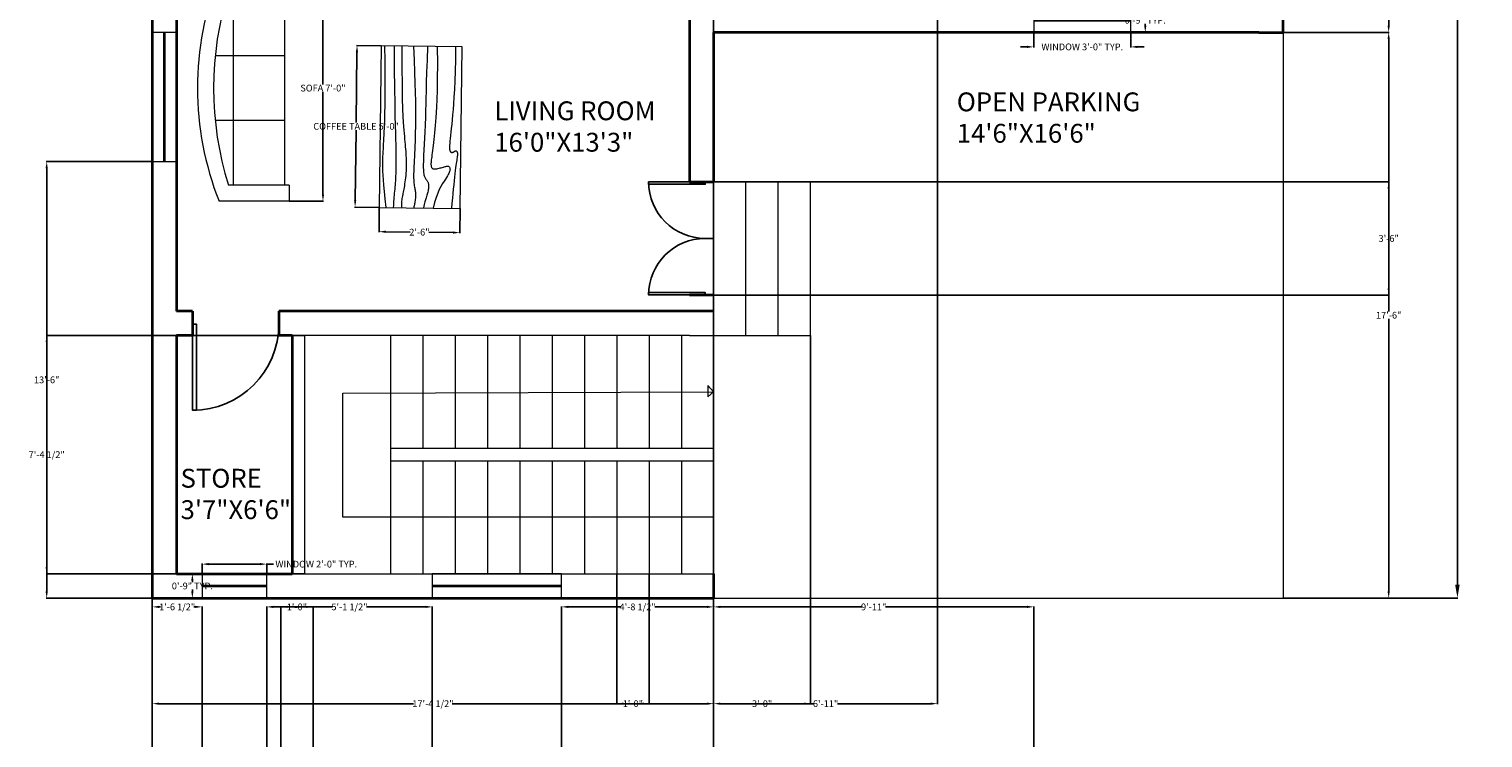
# Model space of a CAD drawing. Units: inches. Extents: x 481 to 2783, y 1975 to 3327.
# Tile 6 of 13: x 1329 to 1869, y 2602 to 2866. Entities that reach past the tile are written whole.
import ezdxf

# ---------------------------------------------------------------- set-up
doc = ezdxf.new("R2010")
doc.units = ezdxf.units.IN
doc.header["$MEASUREMENT"] = 0
for name, color, linetype, lineweight in [('A-ANNO-DIMS', 50, 'Continuous', 18), ('A-AREA-IDEN', 50, 'Continuous', 18), ('A-FLOR-PRKG', 8, 'Continuous', 18), ('A-FURN', 61, 'Continuous', 18), ('A-WALL', 40, 'Continuous', 35), ('DOORS', 10, 'Continuous', 25), ('STAIRCASE', 90, 'Continuous', 18), ('WINDOWS', 220, 'Continuous', 20)]:
    doc.layers.add(name, color=color, linetype=linetype, lineweight=lineweight)
doc.styles.get("Standard").update_dxf_attribs({"font": 'arial.ttf'})
doc.dimstyles.get("Standard").update_dxf_attribs({"dimtxt": 2.5, "dimasz": 2.5, "dimexe": 0.18, "dimexo": 0.0625, "dimgap": 0.09, "dimtad": 0, "dimtih": 1, "dimtoh": 1, "dimzin": 0, "dimdsep": 46, "dimlunit": 3, "dimtxsty": 'Standard', "dimcen": 0.09, "dimadec": 0, "dimazin": 0, "dimtfac": 1, "dimtofl": 0, "dimtmove": 0, "dimatfit": 3, "dimfxl": 1, "dimtolj": 1, "dimtzin": 0, "dimarcsym": 0})

# ---------------------------------------------------------------- blocks, each defined once
blk = doc.blocks.new('*U2')
for p, q in [((0, 0), (0, -6)), ((40, 0), (40, -6))]:
    blk.add_line(p, q)
blk.add_lwpolyline([(0, 0), (0, 40), (1.75, 40), (1.75, 0)], close=True)
blk.add_arc((0, 0), 40, 0, 90)
blk = doc.blocks.new('Sofa - Roundback 7 ft.')
for p, q in [((-12.00002, -32.4421), (-12.00003, -6.5971)), ((11.99997, -32.4421), (11.99998, -6.5971)), ((-36.000027, -34), (-36.000027, -11.4696)), ((-35.999844, -13.3819), (35.9998, -13.3819)), ((35.99998, -34), (35.99998, -11.4696)), ((-36.000027, -32.4421), (35.99998, -32.4421))]:
    blk.add_line(p, q)
for points in [[(-36.000027, -34), (-42.000027, -34), (-42.000027, -8)], [(41.99998, -8), (41.99998, -34), (35.99998, -34)]]:
    blk.add_lwpolyline(points)
for centre, radius, start, end in [((0, -114.25), 114.25, 68.43141, 111.5686), ((-0.00001, -127.1968), 121.1968, 72.72033, 107.2797)]:
    blk.add_arc(centre, radius, start, end)
blk = doc.blocks.new('Table - Rectangular Woodgrain 60 x 30 in.')
for p, q in [((0, 0), (0, -30)), ((60, 0), (0, 0)), ((60, -30), (60, 0)), ((0, -30), (60, -30))]:
    blk.add_line(p, q)
for points in [[(0, -2.4), (4.8155, -2.418), (9.0302, -2.4688), (12.709, -2.5477), (15.9167, -2.65), (18.7181, -2.7711), (21.1781, -2.9063), (23.3616, -3.0508), (25.3333, -3.2), (27.1477, -3.3495), (28.8172, -3.4958), (30.3437, -3.636), (31.7291, -3.7667), (32.9756, -3.8849), (34.0849, -3.9875), (35.059, -4.0714), (35.9, -4.1334), (36.6114, -4.1711), (37.2041, -4.1854), (37.6906, -4.1779), (38.0833, -4.15), (38.3948, -4.1034), (38.6375, -4.0396), (38.8239, -3.9602), (38.9666, -3.8667), (39.0764, -3.7608), (39.1573, -3.6448), (39.2116, -3.521), (39.2416, -3.3917), (39.2498, -3.2593), (39.2385, -3.1261), (39.21, -2.9944), (39.1666, -2.8667), (39.111, -2.7447), (39.0468, -2.6281), (38.978, -2.5163), (38.9083, -2.4083), (38.8418, -2.3035), (38.7823, -2.201), (38.7337, -2.1001), (38.7, -2), (38.6844, -1.9003), (38.6875, -1.8021), (38.7094, -1.707), (38.75, -1.6167), (38.8094, -1.5326), (38.8875, -1.4563), (38.9844, -1.3893), (39.1, -1.3333), (39.2351, -1.2896), (39.3937, -1.2583), (39.5804, -1.2396), (39.8, -1.2333), (40.057, -1.2396), (40.3562, -1.2583), (40.7023, -1.2896), (41.1, -1.3333), (41.5547, -1.3895), (42.0755, -1.4573), (42.6721, -1.5361), (43.3542, -1.625), (44.1316, -1.7233), (45.014, -1.8302), (46.0114, -1.9449), (47.1333, -2.0667), (48.3862, -2.1947), (49.7625, -2.3281), (51.2513, -2.4663), (52.8416, -2.6083), (54.5226, -2.7535), (56.2833, -2.9011), (58.1127, -3.0501), (60, -3.2)], [(0, -9.2), (6.5759, -9.0858), (11.9385, -9.0365), (16.2527, -9.0418), (19.6833, -9.0917), (22.3952, -9.1759), (24.5531, -9.2844), (26.322, -9.4069), (27.8666, -9.5333), (29.3241, -9.6553), (30.7203, -9.7719), (32.0532, -9.8837), (33.3208, -9.9917), (34.5213, -10.0965), (35.6526, -10.199), (36.7128, -10.2999), (37.7, -10.4), (38.6129, -10.4996), (39.4531, -10.5969), (40.223, -10.6895), (40.925, -10.775), (41.5613, -10.8512), (42.1344, -10.9156), (42.6465, -10.966), (43.1, -11), (43.4976, -11.0158), (43.8437, -11.0136), (44.143, -10.9942), (44.4, -10.9583), (44.6195, -10.9069), (44.8062, -10.8406), (44.9648, -10.7603), (45.1, -10.6667), (45.2155, -10.5598), (45.3114, -10.4365), (45.3871, -10.2929), (45.4416, -10.125), (45.4743, -9.929), (45.4844, -9.7011), (45.4709, -9.4371), (45.4333, -9.1333), (45.3716, -8.7883), (45.2896, -8.4104), (45.1919, -8.0107), (45.0833, -7.6), (44.9685, -7.1893), (44.8521, -6.7896), (44.7388, -6.4117), (44.6333, -6.0667), (44.54, -5.7628), (44.4614, -5.4979), (44.4001, -5.2675), (44.3583, -5.0667), (44.3384, -4.8909), (44.3427, -4.7354), (44.3736, -4.5956), (44.4333, -4.4667), (44.5236, -4.3453), (44.6427, -4.2333), (44.7884, -4.1339), (44.9583, -4.05), (45.1501, -3.9849), (45.3614, -3.9417), (45.59, -3.9234), (45.8333, -3.9333), (46.0915, -3.9749), (46.3734, -4.0531), (46.6906, -4.1736), (47.0542, -4.3417), (47.4756, -4.5629), (47.9661, -4.8427), (48.5372, -5.1866), (49.2, -5.6), (49.9676, -6.0844), (50.8594, -6.625), (51.8965, -7.2031), (53.1, -7.8), (54.491, -8.3969), (56.0906, -8.975), (57.9199, -9.5156), (60, -10)], [(0, -12.8), (5.1847, -12.9322), (9.6213, -13.0323), (13.3963, -13.1059), (16.5958, -13.1583), (19.3063, -13.1952), (21.614, -13.2219), (23.6054, -13.2439), (25.3666, -13.2667), (26.9728, -13.2947), (28.4531, -13.3281), (29.8256, -13.3663), (31.1083, -13.4083), (32.3191, -13.4535), (33.476, -13.501), (34.597, -13.5501), (35.7, -13.6), (36.7984, -13.6497), (37.8875, -13.6979), (38.9578, -13.743), (40, -13.7833), (41.0047, -13.8174), (41.9625, -13.8438), (42.864, -13.8607), (43.7, -13.8667), (44.4631, -13.8604), (45.1552, -13.8417), (45.7801, -13.8104), (46.3416, -13.7667), (46.8439, -13.7104), (47.2906, -13.6417), (47.6858, -13.5604), (48.0333, -13.4667), (48.3375, -13.3608), (48.6042, -13.2448), (48.8396, -13.121), (49.05, -12.9917), (49.2417, -12.8593), (49.4208, -12.7261), (49.5937, -12.5944), (49.7667, -12.4667), (49.9452, -12.3451), (50.1323, -12.2313), (50.3303, -12.1268), (50.5416, -12.0333), (50.7686, -11.9524), (51.0135, -11.8854), (51.2788, -11.8341), (51.5666, -11.8), (51.8785, -11.7843), (52.2116, -11.7865), (52.562, -11.8059), (52.926, -11.8417), (53.2998, -11.8931), (53.6795, -11.9594), (54.0614, -12.0397), (54.4416, -12.1333), (54.8223, -12.2401), (55.2293, -12.3625), (55.6942, -12.5037), (56.2489, -12.6667), (56.9251, -12.8547), (57.7545, -13.0708), (58.7689, -13.3182), (60, -13.6)], [(0, -18), (5.124, -17.7273), (9.6609, -17.5057), (13.6705, -17.3303), (17.2125, -17.1958), (20.3467, -17.0973), (23.1328, -17.0297), (25.6307, -16.9878), (27.9, -16.9667), (29.9928, -16.9617), (31.9302, -16.9703), (33.7254, -16.9907), (35.3917, -17.0208), (36.9423, -17.0588), (38.3906, -17.1026), (39.7499, -17.1503), (41.0333, -17.2), (42.2519, -17.2496), (43.4073, -17.2969), (44.4986, -17.3395), (45.525, -17.375), (46.4858, -17.4012), (47.3802, -17.4156), (48.2074, -17.416), (48.9667, -17.4), (49.6583, -17.3662), (50.2872, -17.3167), (50.8595, -17.2547), (51.3812, -17.1833), (51.8584, -17.1057), (52.2971, -17.025), (52.7034, -16.9443), (53.0833, -16.8667), (53.443, -16.7951), (53.789, -16.7313), (54.128, -16.6768), (54.4666, -16.6334), (54.8115, -16.6024), (55.1693, -16.5854), (55.5465, -16.5841), (55.95, -16.6), (56.3828, -16.6337), (56.8346, -16.6823), (57.2915, -16.7418), (57.7396, -16.8084), (58.165, -16.878), (58.5539, -16.9469), (58.8924, -17.0111), (59.1666, -17.0667), (59.3679, -17.1107), (59.5078, -17.1438), (59.6032, -17.1675), (59.6708, -17.1833), (59.7275, -17.193), (59.7901, -17.1979), (59.8753, -17.1998), (60, -17.2)], [(0, -22.4), (8.0098, -22.2501), (14.4094, -22.1011), (19.4168, -21.9535), (23.25, -21.8083), (26.1269, -21.6663), (28.2656, -21.5281), (29.884, -21.3947), (31.2, -21.2667), (32.3967, -21.1448), (33.5172, -21.0292), (34.5697, -20.9198), (35.5625, -20.8167), (36.5037, -20.7198), (37.4015, -20.6292), (38.2642, -20.5448), (39.1, -20.4667), (39.9164, -20.3951), (40.7187, -20.3313), (41.5117, -20.2768), (42.3, -20.2333), (43.0883, -20.2024), (43.8812, -20.1854), (44.6836, -20.1841), (45.5, -20.2), (46.3328, -20.234), (47.1747, -20.2844), (48.0163, -20.3488), (48.8479, -20.425), (49.66, -20.5106), (50.4429, -20.6031), (51.1872, -20.7004), (51.8833, -20.8), (52.5246, -20.8999), (53.1166, -20.9995), (53.6681, -21.0983), (54.1875, -21.1958), (54.6834, -21.2919), (55.1646, -21.3859), (55.6394, -21.4777), (56.1167, -21.5667), (56.6028, -21.6515), (57.0961, -21.7266), (57.5929, -21.7852), (58.0896, -21.8208), (58.5823, -21.8268), (59.0674, -21.7964), (59.5412, -21.723), (60, -21.6)], [(0, -25.2), (8.6355, -25.0504), (15.7026, -24.9031), (21.4049, -24.7606), (25.9458, -24.625), (29.529, -24.4988), (32.3578, -24.3844), (34.6359, -24.284), (36.5667, -24.2), (38.3213, -24.1341), (39.9417, -24.0854), (41.437, -24.0523), (42.8167, -24.0333), (44.0901, -24.0268), (45.2667, -24.0313), (46.3557, -24.0451), (47.3667, -24.0667), (48.309, -24.0947), (49.1928, -24.1287), (50.0284, -24.168), (50.826, -24.2125), (51.5959, -24.2617), (52.3483, -24.3151), (53.0935, -24.3725), (53.8417, -24.4334), (54.6009, -24.497), (55.3699, -24.561), (56.1454, -24.6226), (56.9239, -24.6792), (57.7021, -24.7279), (58.4764, -24.7662), (59.2435, -24.7911), (60, -24.8)], [(0, -28.8), (5.6867, -28.6681), (10.45, -28.5698), (14.407, -28.5012), (17.675, -28.4584), (20.3711, -28.4374), (22.6125, -28.4344), (24.5164, -28.4455), (26.2, -28.4667), (27.762, -28.4947), (29.2276, -28.5281), (30.6033, -28.5663), (31.8958, -28.6084), (33.1118, -28.6535), (34.2578, -28.7011), (35.3405, -28.7501), (36.3666, -28.8), (37.3443, -28.8497), (38.288, -28.8974), (39.2137, -28.9412), (40.1375, -28.9792), (41.0753, -29.0093), (42.0432, -29.0297), (43.0572, -29.0384), (44.1333, -29.0333), (45.2936, -29.0114), (46.5843, -28.9641), (48.0579, -28.8816), (49.7666, -28.7542), (51.7629, -28.5721), (54.0989, -28.3255), (56.8272, -28.0048), (60, -27.6)]]:
    blk.add_lwpolyline(points)
blk = doc.blocks.new('*D23')
at = {"layer": 'A-ANNO-DIMS', "color": 0, "lineweight": -2, "transparency": 16777216}
for p, q in [((1794.5, 3254.32), (1859.35, 3254.32)), ((1859.17, 3249.32), (1859.17, 2959.52)), ((1859.17, 2659.32), (1859.17, 2949.13)), ((1794.5, 2654.32), (1859.35, 2654.32))]:
    blk.add_line(p, q, dxfattribs=at)
at = {"layer": 'A-ANNO-DIMS', "color": 0, "transparency": 16777216}
for points in [[(1858.33, 3249.32), (1860, 3249.32), (1859.17, 3254.32)], [(1858.33, 2659.32), (1860, 2659.32), (1859.17, 2654.32)]]:
    blk.add_solid(points, dxfattribs=at)
at = {"layer": 'Defpoints', "color": 0, "transparency": 16777216}
for p in [(1794.44, 3254.32), (1794.44, 2654.32), (1859.17, 2654.32)]:
    blk.add_point(p, dxfattribs=at)
at = {"layer": 'A-ANNO-DIMS', "color": 0, "transparency": 16777216, "insert": (1859.17, 2954.32), "char_height": 10, "attachment_point": 5}
blk.add_mtext("\\A1;50'", dxfattribs=at)
blk = doc.blocks.new('WIN-PLAN-48IN')
for p, q in [((0, 4.75), (48, 4.75)), ((0, 4.25), (48, 4.25))]:
    blk.add_line(p, q)
blk.add_lwpolyline([(0, 0), (48, 0), (48, 9), (0, 9)], close=True)
blk = doc.blocks.new('WIN-PLAN-36IN')
for p, q in [((0, 4.75), (36, 4.75)), ((0, 4.25), (36, 4.25))]:
    blk.add_line(p, q)
blk.add_lwpolyline([(0, 0), (36, 0), (36, 9), (0, 9)], close=True)
blk = doc.blocks.new('WIN-PLAN-24IN')
for p, q in [((0, 4.75), (24, 4.75)), ((0, 4.25), (24, 4.25))]:
    blk.add_line(p, q)
blk.add_lwpolyline([(0, 0), (24, 0), (24, 9), (0, 9)], close=True)
blk = doc.blocks.new('*D30')
at = {"layer": 'A-ANNO-DIMS', "color": 0, "lineweight": -2, "transparency": 16777216}
for p, q in [((1701.84, 2864.26), (1701.84, 2858.74)), ((1737.84, 2864.26), (1737.84, 2858.74)), ((1699.34, 2858.92), (1696.84, 2858.92)), ((1740.34, 2858.92), (1742.84, 2858.92))]:
    blk.add_line(p, q, dxfattribs=at)
at = {"layer": 'A-ANNO-DIMS', "color": 0, "transparency": 16777216}
for points in [[(1699.34, 2859.34), (1699.34, 2858.51), (1701.84, 2858.92)], [(1740.34, 2859.34), (1740.34, 2858.51), (1737.84, 2858.92)]]:
    blk.add_solid(points, dxfattribs=at)
at = {"layer": 'Defpoints', "color": 0, "transparency": 16777216}
for p in [(1701.84, 2864.32), (1737.84, 2864.32), (1737.84, 2858.92)]:
    blk.add_point(p, dxfattribs=at)
at = {"layer": 'A-ANNO-DIMS', "color": 0, "transparency": 16777216, "insert": (1719.84, 2858.92), "char_height": 2.5, "attachment_point": 5}
blk.add_mtext('\\A1;WINDOW 3\'-0" TYP.', dxfattribs=at)
blk = doc.blocks.new('*D31')
at = {"layer": 'A-ANNO-DIMS', "color": 0, "lineweight": -2, "transparency": 16777216}
for p, q in [((1737.9, 2873.32), (1743.42, 2873.32)), ((1743.24, 2870.82), (1743.24, 2870.19)), ((1743.24, 2866.82), (1743.24, 2867.46)), ((1737.9, 2864.32), (1743.42, 2864.32))]:
    blk.add_line(p, q, dxfattribs=at)
at = {"layer": 'A-ANNO-DIMS', "color": 0, "transparency": 16777216}
for points in [[(1742.83, 2870.82), (1743.66, 2870.82), (1743.24, 2873.32)], [(1742.83, 2866.82), (1743.66, 2866.82), (1743.24, 2864.32)]]:
    blk.add_solid(points, dxfattribs=at)
at = {"layer": 'Defpoints', "color": 0, "transparency": 16777216}
for p in [(1737.84, 2873.32), (1743.24, 2873.32), (1737.84, 2864.32)]:
    blk.add_point(p, dxfattribs=at)
at = {"layer": 'A-ANNO-DIMS', "color": 0, "transparency": 16777216, "insert": (1743.24, 2868.82), "char_height": 2.5, "attachment_point": 5}
blk.add_mtext('\\A1;0\'-9" TYP.', dxfattribs=at)
blk = doc.blocks.new('*D32')
at = {"layer": 'A-ANNO-DIMS', "color": 0, "lineweight": -2, "transparency": 16777216}
for p, q in [((1392.94, 2663.39), (1392.94, 2667.1)), ((1395.44, 2666.92), (1414.44, 2666.92)), ((1416.94, 2663.39), (1416.94, 2667.1)), ((1416.94, 2666.92), (1419.44, 2666.92))]:
    blk.add_line(p, q, dxfattribs=at)
at = {"layer": 'A-ANNO-DIMS', "color": 0, "transparency": 16777216}
for points in [[(1395.44, 2667.34), (1395.44, 2666.51), (1392.94, 2666.92)], [(1414.44, 2667.34), (1414.44, 2666.51), (1416.94, 2666.92)]]:
    blk.add_solid(points, dxfattribs=at)
at = {"layer": 'Defpoints', "color": 0, "transparency": 16777216}
for p in [(1392.94, 2663.32), (1416.94, 2666.92), (1416.94, 2663.32)]:
    blk.add_point(p, dxfattribs=at)
at = {"layer": 'A-ANNO-DIMS', "color": 0, "transparency": 16777216, "insert": (1435.35, 2666.92), "char_height": 2.5, "attachment_point": 5}
blk.add_mtext('\\A1;WINDOW 2\'-0" TYP.', dxfattribs=at)
blk = doc.blocks.new('*D33')
at = {"layer": 'A-ANNO-DIMS', "color": 0, "lineweight": -2, "transparency": 16777216}
for p, q in [((1392.88, 2663.32), (1389.16, 2663.32)), ((1389.34, 2660.82), (1389.34, 2660.19)), ((1389.34, 2656.82), (1389.34, 2657.46)), ((1392.88, 2654.32), (1389.16, 2654.32))]:
    blk.add_line(p, q, dxfattribs=at)
at = {"layer": 'A-ANNO-DIMS', "color": 0, "transparency": 16777216}
for points in [[(1388.92, 2660.82), (1389.75, 2660.82), (1389.34, 2663.32)], [(1388.92, 2656.82), (1389.75, 2656.82), (1389.34, 2654.32)]]:
    blk.add_solid(points, dxfattribs=at)
at = {"layer": 'Defpoints', "color": 0, "transparency": 16777216}
for p in [(1389.34, 2663.32), (1392.94, 2663.32), (1392.94, 2654.32)]:
    blk.add_point(p, dxfattribs=at)
at = {"layer": 'A-ANNO-DIMS', "color": 0, "transparency": 16777216, "insert": (1389.34, 2658.82), "char_height": 2.5, "attachment_point": 5}
blk.add_mtext('\\A1;0\'-9" TYP.', dxfattribs=at)
blk = doc.blocks.new('*D44')
at = {"layer": 'A-ANNO-DIMS', "color": 0, "lineweight": -2, "transparency": 16777216}
for p, q in [((1425.31, 2885.62), (1438.02, 2885.62)), ((1437.84, 2883.12), (1437.84, 2845)), ((1437.84, 2804.12), (1437.84, 2842.24)), ((1425.31, 2801.62), (1438.02, 2801.62))]:
    blk.add_line(p, q, dxfattribs=at)
at = {"layer": 'A-ANNO-DIMS', "color": 0, "transparency": 16777216}
for points in [[(1437.43, 2883.12), (1438.26, 2883.12), (1437.84, 2885.62)], [(1437.43, 2804.12), (1438.26, 2804.12), (1437.84, 2801.62)]]:
    blk.add_solid(points, dxfattribs=at)
at = {"layer": 'Defpoints', "color": 0, "transparency": 16777216}
for p in [(1425.24, 2885.62), (1437.84, 2885.62), (1425.24, 2801.62)]:
    blk.add_point(p, dxfattribs=at)
at = {"layer": 'A-ANNO-DIMS', "color": 0, "transparency": 16777216, "insert": (1437.84, 2843.62), "char_height": 2.5, "attachment_point": 5}
blk.add_mtext('\\A1;SOFA 7\'-0"', dxfattribs=at)
blk = doc.blocks.new('*D48')
at = {"layer": 'A-ANNO-DIMS', "color": 0, "lineweight": -2, "transparency": 16777216}
for p, q in [((1450.47, 2856.93), (1450.15, 2830.82)), ((1459.43, 2859.32), (1450.32, 2859.43)), ((1449.8, 2801.94), (1450.12, 2828.05)), ((1458.71, 2799.33), (1449.59, 2799.44))]:
    blk.add_line(p, q, dxfattribs=at)
at = {"layer": 'A-ANNO-DIMS', "color": 0, "transparency": 16777216}
for points in [[(1450.05, 2856.94), (1450.88, 2856.93), (1450.5, 2859.43)], [(1449.39, 2801.94), (1450.22, 2801.93), (1449.77, 2799.44)]]:
    blk.add_solid(points, dxfattribs=at)
at = {"layer": 'Defpoints', "color": 0, "transparency": 16777216}
for p in [(1459.5, 2859.32), (1449.77, 2799.44), (1458.77, 2799.33)]:
    blk.add_point(p, dxfattribs=at)
at = {"layer": 'A-ANNO-DIMS', "color": 0, "transparency": 16777216, "insert": (1450.14, 2829.43), "char_height": 2.5, "attachment_point": 5}
blk.add_mtext('\\A1;COFFEE TABLE 5\'-0"', dxfattribs=at)
blk = doc.blocks.new('*D49')
at = {"layer": 'A-ANNO-DIMS', "color": 0, "lineweight": -2, "transparency": 16777216}
for p, q in [((1458.77, 2799.27), (1458.66, 2790.15)), ((1488.77, 2798.9), (1488.66, 2789.79)), ((1461.16, 2790.3), (1470.23, 2790.19)), ((1486.16, 2790), (1477.1, 2790.11))]:
    blk.add_line(p, q, dxfattribs=at)
at = {"layer": 'A-ANNO-DIMS', "color": 0, "transparency": 16777216}
for points in [[(1461.17, 2790.72), (1461.16, 2789.88), (1458.67, 2790.33)], [(1486.17, 2790.41), (1486.16, 2789.58), (1488.66, 2789.97)]]:
    blk.add_solid(points, dxfattribs=at)
at = {"layer": 'Defpoints', "color": 0, "transparency": 16777216}
for p in [(1458.77, 2799.33), (1488.77, 2798.97), (1488.66, 2789.97)]:
    blk.add_point(p, dxfattribs=at)
at = {"layer": 'A-ANNO-DIMS', "color": 0, "transparency": 16777216, "insert": (1473.66, 2790.15), "char_height": 2.5, "attachment_point": 5}
blk.add_mtext('\\A1;2\'-6"', dxfattribs=at)
blk = doc.blocks.new('*D76')
at = {"layer": 'A-ANNO-DIMS', "color": 0, "lineweight": -2, "transparency": 16777216}
for p, q in [((1374.44, 2276.88), (1374.44, 2651.23)), ((1392.94, 2253.88), (1392.94, 2651.23)), ((1376.94, 2651.05), (1377.48, 2651.05)), ((1390.44, 2651.05), (1389.9, 2651.05))]:
    blk.add_line(p, q, dxfattribs=at)
at = {"layer": 'A-ANNO-DIMS', "color": 0, "transparency": 16777216}
for points in [[(1376.94, 2651.47), (1376.94, 2650.64), (1374.44, 2651.05)], [(1390.44, 2651.47), (1390.44, 2650.64), (1392.94, 2651.05)]]:
    blk.add_solid(points, dxfattribs=at)
at = {"layer": 'Defpoints', "color": 0, "transparency": 16777216}
for p in [(1392.94, 2651.05), (1374.44, 2276.82), (1392.94, 2253.82)]:
    blk.add_point(p, dxfattribs=at)
at = {"layer": 'A-ANNO-DIMS', "color": 0, "transparency": 16777216, "insert": (1383.69, 2651.05), "char_height": 2.5, "attachment_point": 5}
blk.add_mtext('\\A1;1\'-6 1/2"', dxfattribs=at)
blk = doc.blocks.new('*D77')
at = {"layer": 'A-ANNO-DIMS', "color": 0, "lineweight": -2, "transparency": 16777216}
for p, q in [((1416.94, 2253.88), (1416.94, 2651.23)), ((1478.44, 2234.88), (1478.44, 2651.23)), ((1419.44, 2651.05), (1441.36, 2651.05)), ((1475.94, 2651.05), (1454.01, 2651.05))]:
    blk.add_line(p, q, dxfattribs=at)
at = {"layer": 'A-ANNO-DIMS', "color": 0, "transparency": 16777216}
for points in [[(1419.44, 2651.47), (1419.44, 2650.64), (1416.94, 2651.05)], [(1475.94, 2651.47), (1475.94, 2650.64), (1478.44, 2651.05)]]:
    blk.add_solid(points, dxfattribs=at)
at = {"layer": 'Defpoints', "color": 0, "transparency": 16777216}
for p in [(1478.44, 2651.05), (1416.94, 2253.82), (1478.44, 2234.82)]:
    blk.add_point(p, dxfattribs=at)
at = {"layer": 'A-ANNO-DIMS', "color": 0, "transparency": 16777216, "insert": (1447.69, 2651.05), "char_height": 2.5, "attachment_point": 5}
blk.add_mtext('\\A1;5\'-1 1/2"', dxfattribs=at)
blk = doc.blocks.new('*D78')
at = {"layer": 'A-ANNO-DIMS', "color": 0, "lineweight": -2, "transparency": 16777216}
for p, q in [((1526.44, 2234.88), (1526.44, 2651.23)), ((1582.94, 2270.88), (1582.94, 2651.23)), ((1528.94, 2651.05), (1548.31, 2651.05)), ((1580.44, 2651.05), (1561.06, 2651.05))]:
    blk.add_line(p, q, dxfattribs=at)
at = {"layer": 'A-ANNO-DIMS', "color": 0, "transparency": 16777216}
for points in [[(1528.94, 2651.47), (1528.94, 2650.64), (1526.44, 2651.05)], [(1580.44, 2651.47), (1580.44, 2650.64), (1582.94, 2651.05)]]:
    blk.add_solid(points, dxfattribs=at)
at = {"layer": 'Defpoints', "color": 0, "transparency": 16777216}
for p in [(1582.94, 2651.05), (1582.94, 2270.82), (1526.44, 2234.82)]:
    blk.add_point(p, dxfattribs=at)
at = {"layer": 'A-ANNO-DIMS', "color": 0, "transparency": 16777216, "insert": (1554.69, 2651.05), "char_height": 2.5, "attachment_point": 5}
blk.add_mtext('\\A1;4\'-8 1/2"', dxfattribs=at)
blk = doc.blocks.new('*D79')
at = {"layer": 'A-ANNO-DIMS', "color": 0, "lineweight": -2, "transparency": 16777216}
for p, q in [((1582.94, 2270.88), (1582.94, 2651.23)), ((1701.84, 2234.88), (1701.84, 2651.23)), ((1585.44, 2651.05), (1638.01, 2651.05)), ((1699.34, 2651.05), (1646.77, 2651.05))]:
    blk.add_line(p, q, dxfattribs=at)
at = {"layer": 'A-ANNO-DIMS', "color": 0, "transparency": 16777216}
for points in [[(1585.44, 2651.47), (1585.44, 2650.64), (1582.94, 2651.05)], [(1699.34, 2651.47), (1699.34, 2650.64), (1701.84, 2651.05)]]:
    blk.add_solid(points, dxfattribs=at)
at = {"layer": 'Defpoints', "color": 0, "transparency": 16777216}
for p in [(1701.84, 2651.05), (1582.94, 2270.82), (1701.84, 2234.82)]:
    blk.add_point(p, dxfattribs=at)
at = {"layer": 'A-ANNO-DIMS', "color": 0, "transparency": 16777216, "insert": (1642.39, 2651.05), "char_height": 2.5, "attachment_point": 5}
blk.add_mtext('\\A1;9\'-11"', dxfattribs=at)
blk = doc.blocks.new('*D81')
at = {"layer": 'A-ANNO-DIMS', "color": 0, "lineweight": -2, "transparency": 16777216}
for p, q in [((1422.16, 2270.88), (1422.16, 2651.23)), ((1434.16, 2270.88), (1434.16, 2651.23)), ((1424.66, 2651.05), (1424.87, 2651.05)), ((1431.66, 2651.05), (1431.46, 2651.05))]:
    blk.add_line(p, q, dxfattribs=at)
at = {"layer": 'A-ANNO-DIMS', "color": 0, "transparency": 16777216}
for points in [[(1424.66, 2651.47), (1424.66, 2650.64), (1422.16, 2651.05)], [(1431.66, 2651.47), (1431.66, 2650.64), (1434.16, 2651.05)]]:
    blk.add_solid(points, dxfattribs=at)
at = {"layer": 'Defpoints', "color": 0, "transparency": 16777216}
for p in [(1434.16, 2651.05), (1422.16, 2270.82), (1434.16, 2270.82)]:
    blk.add_point(p, dxfattribs=at)
at = {"layer": 'A-ANNO-DIMS', "color": 0, "transparency": 16777216, "insert": (1428.16, 2651.05), "char_height": 2.5, "attachment_point": 5}
blk.add_mtext('\\A1;1\'-0"', dxfattribs=at)
blk = doc.blocks.new('*D86')
at = {"layer": 'A-ANNO-DIMS', "color": 0, "lineweight": -2, "transparency": 16777216}
for p, q in [((1374.44, 2654.26), (1374.44, 2614.94)), ((1582.94, 2654.26), (1582.94, 2614.94)), ((1376.94, 2615.12), (1471.51, 2615.12)), ((1580.44, 2615.12), (1485.87, 2615.12))]:
    blk.add_line(p, q, dxfattribs=at)
at = {"layer": 'A-ANNO-DIMS', "color": 0, "transparency": 16777216}
for points in [[(1376.94, 2615.54), (1376.94, 2614.71), (1374.44, 2615.12)], [(1580.44, 2615.54), (1580.44, 2614.71), (1582.94, 2615.12)]]:
    blk.add_solid(points, dxfattribs=at)
at = {"layer": 'Defpoints', "color": 0, "transparency": 16777216}
for p in [(1374.44, 2654.32), (1582.94, 2654.32), (1582.94, 2615.12)]:
    blk.add_point(p, dxfattribs=at)
at = {"layer": 'A-ANNO-DIMS', "color": 0, "transparency": 16777216, "insert": (1478.69, 2615.12), "char_height": 2.5, "attachment_point": 5}
blk.add_mtext('\\A1;17\'-4 1/2"', dxfattribs=at)
blk = doc.blocks.new('*D87')
at = {"layer": 'A-ANNO-DIMS', "color": 0, "lineweight": -2, "transparency": 16777216}
for p, q in [((1794.5, 2864.32), (1833.82, 2864.32)), ((1833.64, 2861.82), (1833.64, 2760.69)), ((1833.64, 2656.82), (1833.64, 2757.96)), ((1794.5, 2654.32), (1833.82, 2654.32))]:
    blk.add_line(p, q, dxfattribs=at)
at = {"layer": 'A-ANNO-DIMS', "color": 0, "transparency": 16777216}
for points in [[(1833.22, 2861.82), (1834.05, 2861.82), (1833.64, 2864.32)], [(1833.22, 2656.82), (1834.05, 2656.82), (1833.64, 2654.32)]]:
    blk.add_solid(points, dxfattribs=at)
at = {"layer": 'Defpoints', "color": 0, "transparency": 16777216}
for p in [(1794.44, 2864.32), (1833.64, 2864.32), (1794.44, 2654.32)]:
    blk.add_point(p, dxfattribs=at)
at = {"layer": 'A-ANNO-DIMS', "color": 0, "transparency": 16777216, "insert": (1833.64, 2759.32), "char_height": 2.5, "attachment_point": 5}
blk.add_mtext('\\A1;17\'-6"', dxfattribs=at)
blk = doc.blocks.new('*D88')
at = {"layer": 'A-ANNO-DIMS', "color": 0, "lineweight": -2, "transparency": 16777216}
for p, q in [((1794.5, 2883.62), (1833.82, 2883.62)), ((1833.64, 2881.12), (1833.64, 2875.35)), ((1833.64, 2866.82), (1833.64, 2872.59)), ((1794.5, 2864.32), (1833.82, 2864.32))]:
    blk.add_line(p, q, dxfattribs=at)
at = {"layer": 'A-ANNO-DIMS', "color": 0, "transparency": 16777216}
for points in [[(1833.22, 2881.12), (1834.05, 2881.12), (1833.64, 2883.62)], [(1833.22, 2866.82), (1834.05, 2866.82), (1833.64, 2864.32)]]:
    blk.add_solid(points, dxfattribs=at)
at = {"layer": 'Defpoints', "color": 0, "transparency": 16777216}
for p in [(1794.44, 2883.62), (1833.64, 2883.62), (1794.44, 2864.32)]:
    blk.add_point(p, dxfattribs=at)
at = {"layer": 'A-ANNO-DIMS', "color": 0, "transparency": 16777216, "insert": (1833.64, 2873.97), "char_height": 2.5, "attachment_point": 5}
blk.add_mtext('\\A1;1\'-7 1/2"', dxfattribs=at)
blk = doc.blocks.new('*D91')
at = {"layer": 'A-ANNO-DIMS', "color": 0, "lineweight": -2, "transparency": 16777216}
for p, q in [((1374.38, 2816.32), (1335.06, 2816.32)), ((1335.24, 2813.82), (1335.24, 2736.69)), ((1335.24, 2656.82), (1335.24, 2733.96)), ((1374.38, 2654.32), (1335.06, 2654.32))]:
    blk.add_line(p, q, dxfattribs=at)
at = {"layer": 'A-ANNO-DIMS', "color": 0, "transparency": 16777216}
for points in [[(1334.82, 2813.82), (1335.65, 2813.82), (1335.24, 2816.32)], [(1334.82, 2656.82), (1335.65, 2656.82), (1335.24, 2654.32)]]:
    blk.add_solid(points, dxfattribs=at)
at = {"layer": 'Defpoints', "color": 0, "transparency": 16777216}
for p in [(1335.24, 2816.32), (1374.44, 2816.32), (1374.44, 2654.32)]:
    blk.add_point(p, dxfattribs=at)
at = {"layer": 'A-ANNO-DIMS', "color": 0, "transparency": 16777216, "insert": (1335.24, 2735.32), "char_height": 2.5, "attachment_point": 5}
blk.add_mtext('\\A1;13\'-6"', dxfattribs=at)
blk = doc.blocks.new('*D93')
at = {"layer": 'A-ANNO-DIMS', "color": 0, "lineweight": -2, "transparency": 16777216}
for p, q in [((1430.88, 2751.82), (1335.06, 2751.82)), ((1335.24, 2749.32), (1335.24, 2708.96)), ((1335.24, 2665.82), (1335.24, 2706.19)), ((1430.88, 2663.32), (1335.06, 2663.32))]:
    blk.add_line(p, q, dxfattribs=at)
at = {"layer": 'A-ANNO-DIMS', "color": 0, "transparency": 16777216}
for points in [[(1334.82, 2749.32), (1335.65, 2749.32), (1335.24, 2751.82)], [(1334.82, 2665.82), (1335.65, 2665.82), (1335.24, 2663.32)]]:
    blk.add_solid(points, dxfattribs=at)
at = {"layer": 'Defpoints', "color": 0, "transparency": 16777216}
for p in [(1335.24, 2751.82), (1430.94, 2751.82), (1430.94, 2663.32)]:
    blk.add_point(p, dxfattribs=at)
at = {"layer": 'A-ANNO-DIMS', "color": 0, "transparency": 16777216, "insert": (1335.24, 2707.57), "char_height": 2.5, "attachment_point": 5}
blk.add_mtext('\\A1;7\'-4 1/2"', dxfattribs=at)
blk = doc.blocks.new('*D94')
at = {"layer": 'A-ANNO-DIMS', "color": 0, "lineweight": -2, "transparency": 16777216}
for p, q in [((1582.94, 2751.76), (1582.94, 2614.94)), ((1618.94, 2751.76), (1618.94, 2614.94)), ((1585.44, 2615.12), (1597.53, 2615.12)), ((1616.44, 2615.12), (1604.35, 2615.12))]:
    blk.add_line(p, q, dxfattribs=at)
at = {"layer": 'A-ANNO-DIMS', "color": 0, "transparency": 16777216}
for points in [[(1585.44, 2615.54), (1585.44, 2614.71), (1582.94, 2615.12)], [(1616.44, 2615.54), (1616.44, 2614.71), (1618.94, 2615.12)]]:
    blk.add_solid(points, dxfattribs=at)
at = {"layer": 'Defpoints', "color": 0, "transparency": 16777216}
for p in [(1582.94, 2751.82), (1618.94, 2751.82), (1618.94, 2615.12)]:
    blk.add_point(p, dxfattribs=at)
at = {"layer": 'A-ANNO-DIMS', "color": 0, "transparency": 16777216, "insert": (1600.94, 2615.12), "char_height": 2.5, "attachment_point": 5}
blk.add_mtext('\\A1;3\'-0"', dxfattribs=at)
blk = doc.blocks.new('*D95')
at = {"layer": 'A-ANNO-DIMS', "color": 0, "lineweight": -2, "transparency": 16777216}
for p, q in [((1583, 2808.82), (1833.82, 2808.82)), ((1833.64, 2806.32), (1833.64, 2789.19)), ((1833.64, 2769.32), (1833.64, 2786.46)), ((1583, 2766.82), (1833.82, 2766.82))]:
    blk.add_line(p, q, dxfattribs=at)
at = {"layer": 'A-ANNO-DIMS', "color": 0, "transparency": 16777216}
for points in [[(1833.22, 2806.32), (1834.05, 2806.32), (1833.64, 2808.82)], [(1833.22, 2769.32), (1834.05, 2769.32), (1833.64, 2766.82)]]:
    blk.add_solid(points, dxfattribs=at)
at = {"layer": 'Defpoints', "color": 0, "transparency": 16777216}
for p in [(1582.94, 2808.82), (1833.64, 2808.82), (1582.94, 2766.82)]:
    blk.add_point(p, dxfattribs=at)
at = {"layer": 'A-ANNO-DIMS', "color": 0, "transparency": 16777216, "insert": (1833.64, 2787.82), "char_height": 2.5, "attachment_point": 5}
blk.add_mtext('\\A1;3\'-6"', dxfattribs=at)
blk = doc.blocks.new('*D100')
at = {"layer": 'A-ANNO-DIMS', "color": 0, "lineweight": -2, "transparency": 16777216}
for p, q in [((1546.94, 2663.26), (1546.94, 2614.94)), ((1558.94, 2663.26), (1558.94, 2614.94)), ((1549.44, 2615.12), (1549.64, 2615.12)), ((1556.44, 2615.12), (1556.23, 2615.12))]:
    blk.add_line(p, q, dxfattribs=at)
at = {"layer": 'A-ANNO-DIMS', "color": 0, "transparency": 16777216}
for points in [[(1549.44, 2615.54), (1549.44, 2614.71), (1546.94, 2615.12)], [(1556.44, 2615.54), (1556.44, 2614.71), (1558.94, 2615.12)]]:
    blk.add_solid(points, dxfattribs=at)
at = {"layer": 'Defpoints', "color": 0, "transparency": 16777216}
for p in [(1546.94, 2663.32), (1558.94, 2663.32), (1558.94, 2615.12)]:
    blk.add_point(p, dxfattribs=at)
at = {"layer": 'A-ANNO-DIMS', "color": 0, "transparency": 16777216, "insert": (1552.94, 2615.12), "char_height": 2.5, "attachment_point": 5}
blk.add_mtext('\\A1;1\'-0"', dxfattribs=at)
blk = doc.blocks.new('*D104')
at = {"layer": 'A-ANNO-DIMS', "color": 0, "lineweight": -2, "transparency": 16777216}
for p, q in [((1666.06, 2897.26), (1666.06, 2614.94)), ((1582.94, 2873.26), (1582.94, 2614.94)), ((1585.44, 2615.12), (1620.11, 2615.12)), ((1663.56, 2615.12), (1628.89, 2615.12))]:
    blk.add_line(p, q, dxfattribs=at)
at = {"layer": 'A-ANNO-DIMS', "color": 0, "transparency": 16777216}
for points in [[(1585.44, 2615.54), (1585.44, 2614.71), (1582.94, 2615.12)], [(1663.56, 2615.54), (1663.56, 2614.71), (1666.06, 2615.12)]]:
    blk.add_solid(points, dxfattribs=at)
at = {"layer": 'Defpoints', "color": 0, "transparency": 16777216}
for p in [(1666.06, 2897.32), (1582.94, 2873.32), (1666.06, 2615.12)]:
    blk.add_point(p, dxfattribs=at)
at = {"layer": 'A-ANNO-DIMS', "color": 0, "transparency": 16777216, "insert": (1624.5, 2615.12), "char_height": 2.5, "attachment_point": 5}
blk.add_mtext('\\A1;6\'-11"', dxfattribs=at)

msp = doc.modelspace()

# ---------------------------------------------------------------- linework, layer by layer
at = {"layer": 'A-FLOR-PRKG'}
for p in [(1794.438, 2864.323), (1582.938, 2654.323)]:
    msp.add_line(p, (1794.438, 2654.323), dxfattribs=at)
at = {"layer": 'A-WALL'}
for p, q in [((1573.938, 2988.823), (1573.938, 2808.823)), ((1383.438, 2919.823), (1383.438, 2760.823)), ((1785.438, 2864.323), (1582.938, 2864.323)), ((1582.938, 2864.323), (1582.938, 2808.823)), ((1785.438, 2864.323), (1794.438, 2864.323)), ((1573.938, 2808.823), (1582.938, 2808.823)), ((1573.938, 2766.823), (1582.938, 2766.823)), ((1389.438, 2760.823), (1383.438, 2760.823)), ((1389.438, 2760.823), (1389.438, 2751.823)), ((1582.938, 2760.823), (1421.438, 2760.823)), ((1421.438, 2760.823), (1421.438, 2751.823)), ((1383.438, 2751.823), (1383.438, 2663.323)), ((1389.438, 2751.823), (1383.438, 2751.823)), ((1426.438, 2751.823), (1421.438, 2751.823)), ((1426.438, 2751.823), (1426.438, 2663.323)), ((1383.438, 2663.323), (1426.438, 2663.323)), ((1582.938, 2663.323), (1582.938, 2654.323))]:
    msp.add_line(p, q, dxfattribs=at)
msp.add_lwpolyline([(1794.438, 2864.323), (1794.438, 3254.323), (1374.438, 3254.323), (1374.438, 2654.323), (1582.938, 2654.323)], dxfattribs=at)
at = {"layer": 'STAIRCASE'}
for p, q in [((1582.938, 2751.823), (1582.938, 2808.823)), ((1582.938, 2808.823), (1618.938, 2808.823)), ((1594.938, 2751.823), (1594.938, 2808.823)), ((1606.938, 2751.823), (1606.938, 2808.823)), ((1618.938, 2751.823), (1618.938, 2808.823)), ((1573.938, 2751.823), (1430.938, 2751.823)), ((1430.938, 2751.823), (1430.938, 2663.323)), ((1462.938, 2751.823), (1462.938, 2709.823)), ((1474.938, 2751.823), (1474.938, 2709.823)), ((1486.938, 2751.823), (1486.938, 2709.823)), ((1498.938, 2751.823), (1498.938, 2709.823)), ((1510.938, 2751.823), (1510.938, 2709.823)), ((1522.938, 2751.823), (1522.938, 2709.823)), ((1534.938, 2751.823), (1534.938, 2709.823)), ((1546.938, 2751.823), (1546.938, 2709.823)), ((1558.938, 2751.823), (1558.938, 2709.823)), ((1570.938, 2751.823), (1570.938, 2709.823)), ((1573.938, 2751.823), (1582.938, 2751.823)), ((1582.938, 2751.823), (1582.938, 2709.823)), ((1582.938, 2751.823), (1618.938, 2751.823)), ((1582.938, 2730.823), (1580.723, 2733.258)), ((1580.723, 2733.258), (1580.723, 2729.033)), ((1445.281, 2730.443), (1582.938, 2730.823)), ((1445.281, 2684.323), (1445.281, 2730.443)), ((1462.938, 2730.492), (1462.938, 2663.323)), ((1580.723, 2729.033), (1582.938, 2730.823)), ((1582.938, 2709.823), (1462.938, 2709.823)), ((1462.938, 2705.323), (1582.938, 2705.323)), ((1474.938, 2705.323), (1474.938, 2663.323)), ((1486.938, 2705.323), (1486.938, 2663.323)), ((1498.938, 2705.323), (1498.938, 2663.323)), ((1510.938, 2705.323), (1510.938, 2663.323)), ((1522.938, 2705.323), (1522.938, 2663.323)), ((1534.938, 2705.323), (1534.938, 2663.323)), ((1546.938, 2705.323), (1546.938, 2663.323)), ((1558.938, 2705.323), (1558.938, 2663.323)), ((1570.938, 2705.323), (1570.938, 2663.323)), ((1582.938, 2705.323), (1582.938, 2663.323)), ((1582.938, 2684.323), (1445.281, 2684.323)), ((1430.938, 2663.323), (1573.938, 2663.323)), ((1573.938, 2663.323), (1582.938, 2663.323))]:
    msp.add_line(p, q, dxfattribs=at)

# ---------------------------------------------------------------- block references
at = {"layer": 'A-FURN'}
for name, p, rotation in [('Sofa - Roundback 7 ft.', (1391.243, 2843.619), 90), ('Table - Rectangular Woodgrain 60 x 30 in.', (1489.495, 2858.962), 269.3094444056914)]:
    msp.add_blockref(name, p, dxfattribs=dict(at, rotation=rotation))
at = {"layer": 'DOORS'}
for p, xscale, yscale, zscale, rotation in [((1579.788, 2808.823), -0.525, 0.525, 0.525, 90), ((1579.788, 2766.823), 0.525, 0.525, 0.525, 90), ((1389.438, 2756.023), -0.8, 0.8, 0.8, 180)]:
    msp.add_blockref('*U2', p, dxfattribs=dict(at, xscale=xscale, yscale=yscale, zscale=zscale, rotation=rotation))
at = {"layer": 'WINDOWS'}
for name, p in [('WIN-PLAN-36IN', (1701.842, 2864.323)), ('WIN-PLAN-24IN', (1392.938, 2654.323)), ('WIN-PLAN-48IN', (1478.438, 2654.323))]:
    msp.add_blockref(name, p, dxfattribs=at)
at = {"layer": 'WINDOWS', "rotation": 89.99999999999991}
msp.add_blockref('WIN-PLAN-48IN', (1383.438, 2816.323), dxfattribs=at)

# ---------------------------------------------------------------- texts
at = {"layer": 'A-AREA-IDEN', "char_height": 7, "attachment_point": 1}
for s, width, insert in [('OPEN PARKING\\P14\'6"X16\'6"', 83.0373, (1673.237, 2842.014)), ('LIVING ROOM\\P16\'0"X13\'3"', 69.01413, (1501.469, 2838.695)), ('STORE\\P3\'7"X6\'6"', 43.33543, (1384.96, 2702.301))]:
    msp.add_mtext_dynamic_manual_height_columns(s, width=width, gutter_width=1, heights=[0], dxfattribs=dict(at, insert=insert))

# ---------------------------------------------------------------- dimensions: what is measured, and where the dimension line sits
at = {"layer": 'A-ANNO-DIMS'}
dim = msp.add_aligned_dim(p1=(1794.438, 3254.323), p2=(1794.438, 2654.323), distance=64.73, dimstyle='Standard', override={"dimtxt": 10, "dimasz": 5, "dimclrd": 0, "dimclre": 0, "dimclrt": 0}, dxfattribs=at)
dim.commit()
dim.dimension.update_dxf_attribs({"geometry": '*D23', "text_midpoint": (1859.168, 2954.323)})
for base, p1, p2, picture, middle in [((1666.058, 2615.123), (1582.938, 2873.323), (1666.058, 2897.323), '*D104', (1624.498, 2615.123)), ((1618.938, 2615.123), (1582.938, 2751.823), (1618.938, 2751.823), '*D94', (1600.938, 2615.123)), ((1558.938, 2615.123), (1546.938, 2663.323), (1558.938, 2663.323), '*D100', (1552.938, 2615.123)), ((1392.938, 2651.053), (1374.438, 2276.821), (1392.938, 2253.821), '*D76', (1383.688, 2651.053)), ((1582.938, 2615.123), (1374.438, 2654.323), (1582.938, 2654.323), '*D86', (1478.688, 2615.123)), ((1478.438, 2651.053), (1416.938, 2253.821), (1478.438, 2234.821), '*D77', (1447.688, 2651.053)), ((1434.162, 2651.053), (1422.162, 2270.821), (1434.162, 2270.821), '*D81', (1428.162, 2651.053)), ((1582.938, 2651.053), (1526.438, 2234.821), (1582.938, 2270.821), '*D78', (1554.688, 2651.053)), ((1701.842, 2651.053), (1582.938, 2270.821), (1701.842, 2234.821), '*D79', (1642.39, 2651.053))]:
    dim = msp.add_linear_dim(base=base, p1=p1, p2=p2, dimstyle='Standard', override={"dimdec": 1, "dimlfac": 1, "dimrnd": 0, "dimzin": 1, "dimdsep": 46, "dimlunit": 4, "dimfrac": 2}, dxfattribs=at)
    dim.commit()
    dim.dimension.update_dxf_attribs({"geometry": picture, "text_midpoint": middle})
for base, p1, p2, angle, text, picture, middle in [((1437.843, 2885.619), (1425.243, 2801.619), (1425.243, 2885.619), 90, 'SOFA <>', '*D44', (1437.843, 2843.619)), ((1743.242, 2873.323), (1737.842, 2864.323), (1737.842, 2873.323), 90, '<> TYP.', '*D31', (1743.242, 2868.823)), ((1449.774, 2799.437), (1459.497, 2859.324), (1458.774, 2799.328), 269.30944, 'COFFEE TABLE <>', '*D48', (1450.136, 2829.435)), ((1389.338, 2663.323), (1392.938, 2654.323), (1392.938, 2663.323), 90, '<> TYP.', '*D33', (1389.338, 2658.823))]:
    dim = msp.add_linear_dim(base=base, p1=p1, p2=p2, angle=angle, text=text, dimstyle='Standard', override={"dimdec": 1, "dimlfac": 1, "dimrnd": 0, "dimzin": 1, "dimdsep": 46, "dimlunit": 4, "dimfrac": 2}, dxfattribs=at)
    dim.commit()
    dim.dimension.update_dxf_attribs({"geometry": picture, "text_midpoint": middle})
for base, p1, p2, angle, picture, middle in [((1833.638, 2883.616), (1794.438, 2864.323), (1794.438, 2883.616), 90, '*D88', (1833.638, 2873.97)), ((1833.638, 2864.323), (1794.438, 2654.323), (1794.438, 2864.323), 90, '*D87', (1833.638, 2759.323)), ((1335.238, 2816.323), (1374.438, 2654.323), (1374.438, 2816.323), 90, '*D91', (1335.238, 2735.323)), ((1833.638, 2808.823), (1582.938, 2766.823), (1582.938, 2808.823), 90, '*D95', (1833.638, 2787.823)), ((1488.663, 2789.967), (1458.774, 2799.328), (1488.771, 2798.967), 359.30944, '*D49', (1473.664, 2790.148)), ((1335.238, 2751.823), (1430.938, 2663.323), (1430.938, 2751.823), 90, '*D93', (1335.238, 2707.573))]:
    dim = msp.add_linear_dim(base=base, p1=p1, p2=p2, angle=angle, dimstyle='Standard', override={"dimdec": 1, "dimlfac": 1, "dimrnd": 0, "dimzin": 1, "dimdsep": 46, "dimlunit": 4, "dimfrac": 2}, dxfattribs=at)
    dim.commit()
    dim.dimension.update_dxf_attribs({"geometry": picture, "text_midpoint": middle})
for base, p1, p2, picture, middle in [((1737.842, 2858.923), (1701.842, 2864.323), (1737.842, 2864.323), '*D30', (1719.842, 2858.923)), ((1416.938, 2666.923), (1392.938, 2663.323), (1416.938, 2663.323), '*D32', (1435.345, 2666.923))]:
    dim = msp.add_linear_dim(base=base, p1=p1, p2=p2, text='WINDOW <> TYP.', dimstyle='Standard', override={"dimdec": 1, "dimlfac": 1, "dimrnd": 0, "dimzin": 1, "dimdsep": 46, "dimlunit": 4, "dimfrac": 2}, dxfattribs=at)
    dim.commit()
    dim.dimension.update_dxf_attribs({"geometry": picture, "text_midpoint": middle})

doc.saveas('drawing.dxf')
